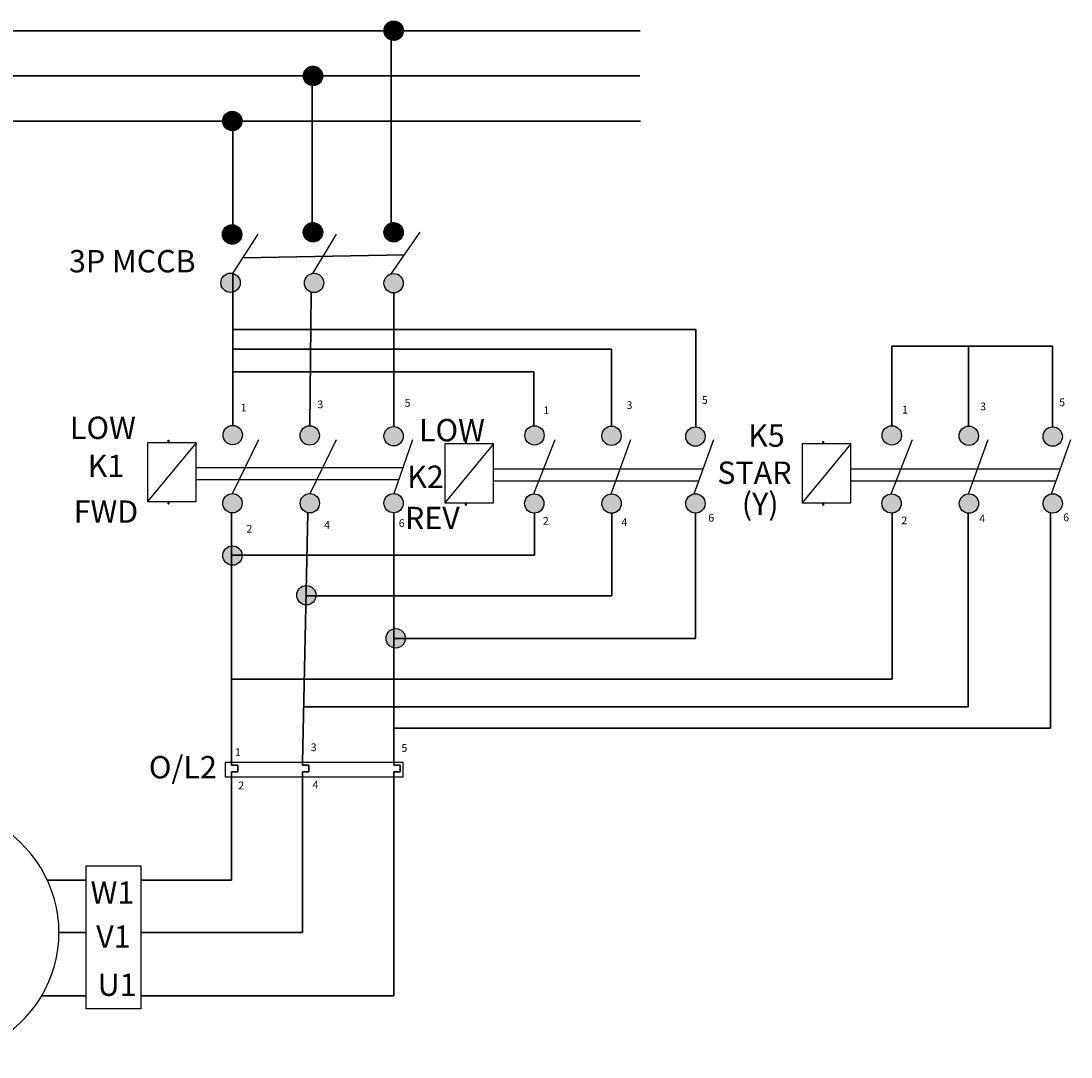
# Model space of a CAD drawing. Units: inches. Extents: x 5169 to 6773, y 5760 to 6563.
# Tile 2 of 2: x 5959 to 6773, y 5760 to 6563. Entities that reach past the tile are written whole.
import ezdxf

# ---------------------------------------------------------------- set-up
doc = ezdxf.new("R2010")
doc.units = ezdxf.units.IN
doc.header["$MEASUREMENT"] = 0
doc.layers.get('0').update_dxf_attribs({"color": 46})
for name, color, linetype, lineweight in [('E-ANNO-TEXT', 2, 'Continuous', 18), ('E-POWR-EQPM', 3, 'Continuous', 25), ('E-POWR-PATT', 8, 'Continuous', 18), ('E-POWR-WIRE', 7, 'Continuous', 35)]:
    doc.layers.add(name, color=color, linetype=linetype, lineweight=lineweight)
doc.styles.get("Standard").update_dxf_attribs({"font": 'arial.ttf'})

# ---------------------------------------------------------------- blocks, each defined once
blk = doc.blocks.new('CONTACTOR-COIL')
blk.add_line((37.69, 45.53), (0, 0))
blk.add_lwpolyline([(0, 0), (37.69, 0), (37.69, 45.53), (0, 45.53)], close=True)

msp = doc.modelspace()

# ---------------------------------------------------------------- hatches: boundary and pattern name
at = {"layer": 'E-POWR-PATT'}
h = msp.add_hatch(dxfattribs=at)
h.set_pattern_fill('ANSI31', color=256)
h.paths.add_polyline_path([(6255.42, 6555.12), (6240.42, 6555.12, -1)])
h.paths.add_polyline_path([(6240.42, 6555.12), (6255.42, 6555.12, -1)])
h.paths.add_polyline_path([(6192.93, 6520.12), (6177.93, 6520.12, -1)])
h.paths.add_polyline_path([(6177.93, 6520.12), (6192.93, 6520.12, -1)])
h.paths.add_polyline_path([(6130.45, 6485.12), (6115.45, 6485.12, -1)])
h.paths.add_polyline_path([(6115.45, 6485.12), (6130.45, 6485.12, -1)])
h = msp.add_hatch(color=256, dxfattribs=at)
h.dxf.hatch_style = 1
h.paths.add_polyline_path([(6255.42, 6359.49, 1), (6240.42, 6359.49, 1)])
h.paths.add_polyline_path([(6192.93, 6398.94, 1), (6177.93, 6398.94, 1)])
h.paths.add_polyline_path([(6255.42, 6398.92, 1), (6240.42, 6398.92, 1)])
h.paths.add_polyline_path([(6130.27, 6397.23, 1), (6115.27, 6397.23, 1)])
h.paths.add_polyline_path([(6193.76, 6359.66, 1), (6178.76, 6359.66, 1)])
h.paths.add_polyline_path([(6129.04, 6359.83, 1), (6114.04, 6359.83, 1)])
h = msp.add_hatch(dxfattribs=at)
h.set_pattern_fill('ANSI31', color=256)
h.paths.add_polyline_path([(6240.42, 6398.92, 1), (6255.42, 6398.92, 1)])
h.paths.add_polyline_path([(6192.93, 6398.94, 1), (6177.93, 6398.94, 1)])
h.paths.add_polyline_path([(6130.27, 6397.23, 1), (6115.27, 6397.23, 1)])
h = msp.add_hatch(color=256, dxfattribs=at)
h.dxf.hatch_style = 1
h.paths.add_polyline_path([(6255.42, 6240.93, 1), (6240.42, 6240.93, 1)])
h.paths.add_polyline_path([(6190.38, 6241.5, 1), (6175.38, 6241.5, 1)])
h.paths.add_polyline_path([(6130.71, 6241.84, 1), (6115.71, 6241.84, 1)])
h = msp.add_hatch(color=256, dxfattribs=at)
h.dxf.hatch_style = 1
h.paths.add_polyline_path([(6489.29, 6240.68, 1), (6474.29, 6240.68, 1)])
h.paths.add_polyline_path([(6364.58, 6241.59, 1), (6349.58, 6241.59, 1)])
h = msp.add_hatch(color=256, dxfattribs=at)
h.dxf.hatch_style = 1
h.paths.add_polyline_path([(6766.15, 6240.68, 1), (6751.15, 6240.68, 1)])
h.paths.add_polyline_path([(6641.44, 6241.59, 1), (6626.44, 6241.59, 1)])
h = msp.add_hatch(color=256, dxfattribs=at)
h.dxf.hatch_style = 1
h.paths.add_polyline_path([(6424.25, 6241.25, 1), (6409.25, 6241.25, 1)])
h = msp.add_hatch(color=256, dxfattribs=at)
h.dxf.hatch_style = 1
h.paths.add_polyline_path([(6701.11, 6241.25, 1), (6686.11, 6241.25, 1)])
h = msp.add_hatch(color=256, dxfattribs=at)
h.dxf.hatch_style = 1
h.paths.add_polyline_path([(6073.81, 6188.53), (6073.23, 6188.53), (6073.23, 6190.4), (6073.81, 6190.4)])
h.paths.add_polyline_path([(6073.79, 6235.92), (6073.21, 6235.92), (6073.21, 6237.79), (6073.79, 6237.79)])
h = msp.add_hatch(color=256, dxfattribs=at)
h.dxf.hatch_style = 1
h.paths.add_polyline_path([(6304.22, 6187.53), (6303.64, 6187.53), (6303.64, 6189.4), (6304.22, 6189.4)])
h.paths.add_polyline_path([(6304.2, 6234.93), (6303.62, 6234.93), (6303.62, 6236.79), (6304.2, 6236.79)])
h = msp.add_hatch(color=256, dxfattribs=at)
h.dxf.hatch_style = 1
h.paths.add_polyline_path([(6581.08, 6187.53), (6580.49, 6187.53), (6580.49, 6189.4), (6581.08, 6189.4)])
h.paths.add_polyline_path([(6581.06, 6234.93), (6580.47, 6234.93), (6580.47, 6236.79), (6581.06, 6236.79)])
h = msp.add_hatch(color=256, dxfattribs=at)
h.dxf.hatch_style = 1
h.paths.add_polyline_path([(6175.49, 6189.04, -1), (6190.49, 6189.04, -1)])
h.paths.add_polyline_path([(6115.53, 6189.04, -0.407395), (6122.86, 6196.54), (6123.21, 6196.54, -0.407395), (6130.53, 6189.04, -1)])
h = msp.add_hatch(color=256, dxfattribs=at)
h.dxf.hatch_style = 1
h.paths.add_polyline_path([(6255.42, 6189.07, -1), (6240.42, 6189.07, -1)])
h.paths.add_polyline_path([(6190.49, 6189.07), (6175.49, 6189.07, -0.996243)])
h = msp.add_hatch(color=256, dxfattribs=at)
h.dxf.hatch_style = 1
h.paths.add_polyline_path([(6409.36, 6188.79, -1), (6424.36, 6188.79, -1)])
h.paths.add_polyline_path([(6349.4, 6188.8, -0.407395), (6356.73, 6196.29), (6357.08, 6196.29, -0.407395), (6364.4, 6188.8, -1)])
h = msp.add_hatch(color=256, dxfattribs=at)
h.dxf.hatch_style = 1
h.paths.add_polyline_path([(6489.29, 6188.82, -1), (6474.29, 6188.82, -1)])
h.paths.add_polyline_path([(6424.36, 6188.82), (6409.36, 6188.82, -0.996243)])
h = msp.add_hatch(color=256, dxfattribs=at)
h.dxf.hatch_style = 1
h.paths.add_polyline_path([(6686.22, 6188.79, -1), (6701.22, 6188.79, -1)])
h.paths.add_polyline_path([(6626.26, 6188.8, -0.407395), (6633.59, 6196.29), (6633.94, 6196.29, -0.407395), (6641.26, 6188.8, -1)])
h = msp.add_hatch(color=256, dxfattribs=at)
h.dxf.hatch_style = 1
h.paths.add_polyline_path([(6766.15, 6188.82, -1), (6751.15, 6188.82, -1)])
h.paths.add_polyline_path([(6701.22, 6188.82), (6686.22, 6188.82, -0.996243)])
h = msp.add_hatch(color=256, dxfattribs=at)
h.dxf.hatch_style = 1
h.paths.add_polyline_path([(6248.04, 6084.34), (6257.05, 6084.34, -0.474651), (6248.04, 6076.99)])
h.paths.add_polyline_path([(6248.04, 6091.69, -0.474651), (6257.05, 6084.34), (6248.04, 6084.34)])
h.paths.add_polyline_path([(6248.04, 6091.69), (6248.04, 6084.34), (6248.04, 6076.99, -0.356253), (6242.05, 6084.34, -0.356253)])
h.paths.add_polyline_path([(6180.06, 6117.23), (6187.81, 6117.23, -0.410427), (6179.91, 6110.26)])
h.paths.add_polyline_path([(6180.24, 6125.24, -0.417716), (6187.82, 6117.74, -0.017058), (6187.81, 6117.23), (6180.06, 6117.23)])
h.paths.add_polyline_path([(6180.24, 6125.24), (6180.06, 6117.23), (6179.91, 6110.26, -0.398114), (6172.82, 6117.74, -0.41072)])
h.paths.add_polyline_path([(6122.23, 6148.87), (6130.52, 6148.87, -0.012478), (6130.53, 6148.49, -0.446102), (6122.23, 6141.04)])
h.paths.add_polyline_path([(6122.23, 6155.95, -0.431224), (6130.52, 6148.87), (6122.23, 6148.87)])
h.paths.add_polyline_path([(6122.23, 6155.95), (6122.23, 6148.87), (6122.23, 6141.04, -0.383028), (6115.53, 6148.49, -0.383028)])

# ---------------------------------------------------------------- linework, layer by layer
at = {"layer": 'E-POWR-EQPM'}
for p, q in [((6123.38, 6367.1), (6142.88, 6397.52)), ((6185.27, 6367.09), (6203.52, 6397.52)), ((6246.09, 6366.76), (6268.58, 6398.94)), ((6073.21, 6235.92), (6073.21, 6237.79)), ((6073.21, 6237.79), (6073.79, 6237.79)), ((6073.79, 6237.79), (6073.79, 6235.92)), ((6123.15, 6196.54), (6143.43, 6238.27)), ((6183.28, 6196.54), (6203.61, 6238.27)), ((6248.43, 6196.55), (6262.86, 6238.27)), ((6303.62, 6234.93), (6303.62, 6236.79)), ((6303.62, 6236.79), (6304.2, 6236.79)), ((6304.2, 6236.79), (6304.2, 6234.93)), ((6356.47, 6196.28), (6373.14, 6238.27)), ((6416.53, 6196.29), (6431.72, 6238.27)), ((6480.73, 6196.25), (6495.95, 6238.27)), ((6580.47, 6234.93), (6580.47, 6236.79)), ((6580.47, 6236.79), (6581.06, 6236.79)), ((6581.06, 6236.79), (6581.06, 6234.93)), ((6633.33, 6196.28), (6650, 6238.27)), ((6693.39, 6196.29), (6708.57, 6238.27)), ((6757.59, 6196.25), (6772.81, 6238.27)), ((6120.67, 6216.41), (6094.83, 6216.41)), ((6255.3, 6216.41), (6116.61, 6216.41)), ((6351.08, 6215.42), (6325.24, 6215.42)), ((6487.67, 6215.42), (6347.02, 6215.42)), ((6627.94, 6215.42), (6602.1, 6215.42)), ((6764.53, 6215.42), (6623.88, 6215.42)), ((6120.67, 6207.12), (6094.83, 6207.12)), ((6252.08, 6207.12), (6120.67, 6207.12)), ((6351.08, 6206.13), (6325.24, 6206.13)), ((6484.31, 6206.13), (6351.08, 6206.13)), ((6627.94, 6206.13), (6602.1, 6206.13)), ((6761.17, 6206.13), (6627.94, 6206.13)), ((6073.23, 6188.53), (6073.23, 6190.4)), ((6073.23, 6188.53), (6073.81, 6188.53)), ((6073.81, 6190.4), (6073.81, 6188.53)), ((6303.64, 6187.53), (6303.64, 6189.4)), ((6303.64, 6187.53), (6304.22, 6187.53)), ((6304.22, 6189.4), (6304.22, 6187.53)), ((6580.49, 6187.53), (6580.49, 6189.4)), ((6580.49, 6187.53), (6581.08, 6187.53)), ((6581.08, 6189.4), (6581.08, 6187.53))]:
    msp.add_line(p, q, dxfattribs=at)
for points in [[(6255.42, 6555.12, -1), (6240.42, 6555.12, -1)], [(6192.93, 6520.12, -1), (6177.93, 6520.12, -1)], [(6130.45, 6485.12, -1), (6115.45, 6485.12, -1)], [(6130.27, 6397.23, -1), (6115.27, 6397.23, -1)], [(6192.93, 6398.94, -1), (6177.93, 6398.94, -1)], [(6255.42, 6398.92, -1), (6240.42, 6398.92, -1)], [(6129.04, 6359.83, -1), (6114.04, 6359.83, -1)], [(6193.76, 6359.66, -1), (6178.76, 6359.66, -1)], [(6255.42, 6359.49, -1), (6240.42, 6359.49, -1)], [(6130.71, 6241.84, -1), (6115.71, 6241.84, -1)], [(6190.38, 6241.5, -1), (6175.38, 6241.5, -1)], [(6364.58, 6241.59, -1), (6349.58, 6241.59, -1)], [(6641.44, 6241.59, -1), (6626.44, 6241.59, -1)], [(6255.42, 6240.93, -1), (6240.42, 6240.93, -1)], [(6424.25, 6241.25, -1), (6409.25, 6241.25, -1)], [(6489.29, 6240.68, -1), (6474.29, 6240.68, -1)], [(6701.11, 6241.25, -1), (6686.11, 6241.25, -1)], [(6766.15, 6240.68, -1), (6751.15, 6240.68, -1)], [(6130.53, 6189.04, -1), (6115.53, 6189.04, -1)], [(6190.49, 6189.04, -1), (6175.49, 6189.04, -1)], [(6255.42, 6189.07, -1), (6240.42, 6189.07, -1)], [(6364.4, 6188.8, -1), (6349.4, 6188.8, -1)], [(6424.36, 6188.79, -1), (6409.36, 6188.79, -1)], [(6489.29, 6188.82, -1), (6474.29, 6188.82, -1)], [(6641.26, 6188.8, -1), (6626.26, 6188.8, -1)], [(6701.22, 6188.79, -1), (6686.22, 6188.79, -1)], [(6766.15, 6188.82, -1), (6751.15, 6188.82, -1)], [(6130.53, 6148.49, -1), (6115.53, 6148.49, -1)], [(6187.82, 6117.74, -1), (6172.82, 6117.74, -1)], [(6257.05, 6084.34, -1), (6242.05, 6084.34, -1)]]:
    msp.add_lwpolyline(points, format="xyb", close=True, dxfattribs=at)
for points in [[(6255.32, 5988.19), (6117.49, 5988.19), (6117.49, 5977.13), (6255.32, 5977.13)], [(6009.6, 5908.17), (6052.08, 5908.17), (6052.08, 5797.38), (6009.6, 5797.38)]]:
    msp.add_lwpolyline(points, close=True, dxfattribs=at)
msp.add_arc((5892.21, 5856.37), 96.38, 266.60656, 93.39344, dxfattribs=at)
at = {"layer": 'E-POWR-WIRE'}
for p, q in [((5317.39, 6555.12), (6439, 6555.12)), ((6246.12, 6547.84), (6246.12, 6406.2)), ((5317.39, 6520.12), (6438.76, 6520.12)), ((6184.67, 6512.66), (6184.67, 6406.4)), ((5317.39, 6485.12), (6439.26, 6485.12)), ((6123.38, 6477.63), (6123.38, 6404.46)), ((6123.38, 6404.46), (6123.38, 6389.76)), ((6256.31, 6381.38), (6131.14, 6379.2)), ((6123.38, 6367.1), (6123.38, 6249.34)), ((6183.99, 6352.51), (6182.92, 6249)), ((6248.04, 6351.99), (6248.04, 6248.43)), ((6123.38, 6323.73), (6454.66, 6323.73)), ((6482.1, 6323.73), (6454.66, 6323.73)), ((6482.1, 6248.18), (6482.1, 6323.73)), ((6123.38, 6308.43), (6416.79, 6308.43)), ((6416.79, 6308.43), (6416.79, 6248.75)), ((6634.04, 6249.09), (6634.04, 6310.76)), ((6634.04, 6310.76), (6693.4, 6310.76)), ((6693.4, 6248.75), (6693.4, 6310.76)), ((6758.37, 6310.76), (6693.4, 6310.76)), ((6758.37, 6248.18), (6758.37, 6310.76)), ((6123.38, 6290.9), (6356.55, 6290.9)), ((6356.55, 6249.07), (6356.55, 6290.9)), ((6122.23, 6181.59), (6122.23, 6031.06)), ((6181.46, 6181.7), (6177.26, 5988.19)), ((6248.04, 6181.57), (6248.04, 5988.19)), ((6356.95, 6181.3), (6356.95, 6148.87)), ((6417.12, 6181.3), (6417.12, 6117.23)), ((6481.91, 6181.32), (6481.91, 6084.34)), ((6634.18, 6181.31), (6634.18, 6052.83)), ((6693.16, 6181.32), (6693.16, 6031.35)), ((6756.9, 6181.53), (6756.9, 6014.85)), ((6356.95, 6148.87), (6122.23, 6148.87)), ((6417.12, 6117.23), (6180.06, 6117.23)), ((6481.91, 6084.34), (6248.04, 6084.34)), ((6122.23, 6052.83), (6634.18, 6052.83)), ((6122.23, 6031.06), (6122.23, 5988.19)), ((6178.2, 6031.35), (6693.16, 6031.35)), ((6248.04, 6014.85), (6756.9, 6014.85)), ((6122.23, 5988.19), (6122.23, 5985.99)), ((6122.23, 5985.99), (6127.23, 5985.99)), ((6127.23, 5980.99), (6122.23, 5980.99)), ((6122.23, 5980.99), (6122.23, 5977.13)), ((6127.23, 5985.99), (6127.23, 5980.99)), ((6177.22, 5985.99), (6177.26, 5988.19)), ((6177.22, 5985.99), (6182.22, 5985.99)), ((6182.22, 5980.99), (6177.22, 5980.99)), ((6177.22, 5980.99), (6177.22, 5977.13)), ((6182.22, 5985.99), (6182.22, 5980.99)), ((6248.04, 5985.99), (6248.04, 5988.19)), ((6248.04, 5985.99), (6253.04, 5985.99)), ((6253.04, 5980.99), (6248.04, 5980.99)), ((6248.04, 5980.99), (6248.04, 5977.13)), ((6253.04, 5985.99), (6253.04, 5980.99)), ((6122.23, 5977.13), (6122.23, 5897.03)), ((6177.22, 5977.13), (6177.22, 5856.37)), ((6248.04, 5977.13), (6248.04, 5807.35)), ((6009.6, 5897.03), (5979.59, 5897.03)), ((6122.23, 5897.03), (6052.08, 5897.03)), ((6009.6, 5856.37), (5988.59, 5856.37)), ((6177.22, 5856.37), (6052.08, 5856.37)), ((6009.6, 5807.35), (5975.2, 5807.35)), ((6248.04, 5807.35), (6052.08, 5807.35))]:
    msp.add_line(p, q, dxfattribs=at)

# ---------------------------------------------------------------- block references
at = {"layer": 'E-POWR-EQPM'}
for p in [(6057.14, 6190.4), (6287.55, 6189.4), (6564.41, 6189.4)]:
    msp.add_blockref('CONTACTOR-COIL', p, dxfattribs=at)

# ---------------------------------------------------------------- texts
at = {"layer": 'E-ANNO-TEXT'}
for s, height, p in [('3P MCCB', 17.303, (5996.35, 6367.88)), ('1', 6.02, (6129.46, 6260.11)), ('3', 6.02, (6188.8, 6262.56)), ('5', 6.02, (6256.39, 6263.78)), ('3', 6.02, (6428.38, 6262.01)), ('5', 6.02, (6486.74, 6265.99)), ('3', 6.02, (6702.43, 6261)), ('5', 6.02, (6763.62, 6264.15)), ('1', 6.02, (6364.03, 6258.02)), ('1', 6.02, (6641.88, 6258.48)), ('LOW', 17.303, (5997.09, 6238.81)), ('LOW', 17.303, (6267.55, 6236.96)), ('K5', 17.303, (6522.61, 6232.75)), ('K1', 17.303, (6010.81, 6209.23)), ('K2', 17.303, (6258.4, 6200.86)), ('STAR', 17.303, (6498.75, 6204.01)), ('(Y)', 17.303, (6517.73, 6179.88)), ('FWD', 17.303, (5999.98, 6173.88)), ('REV', 17.303, (6256.69, 6168.92)), ('6', 6.02, (6251.9, 6170.63)), ('2', 6.02, (6363.53, 6172.3)), ('4', 6.02, (6424.39, 6171.3)), ('6', 6.02, (6491.73, 6174.79)), ('2', 6.02, (6641.31, 6172.7)), ('4', 6.02, (6701.74, 6174.1)), ('6', 6.02, (6766.75, 6175.09)), ('2', 6.02, (6133.81, 6166.21)), ('4', 6.02, (6193.99, 6169.14)), ('1', 6.02, (6124.91, 5993.08)), ('3', 6.02, (6183.64, 5996.93)), ('5', 6.02, (6253.92, 5996.33)), ('O/L2', 17.303, (6058.24, 5975.84)), ('2', 6.02, (6127.5, 5967.35)), ('4', 6.02, (6185.11, 5967.97)), ('W1', 17.303, (6013.04, 5878.69)), ('V1', 17.303, (6017.4, 5844.6)), ('U1', 17.303, (6018.54, 5807.35))]:
    msp.add_text(s, height=height, dxfattribs=at).set_placement(p)

doc.saveas('drawing.dxf')
